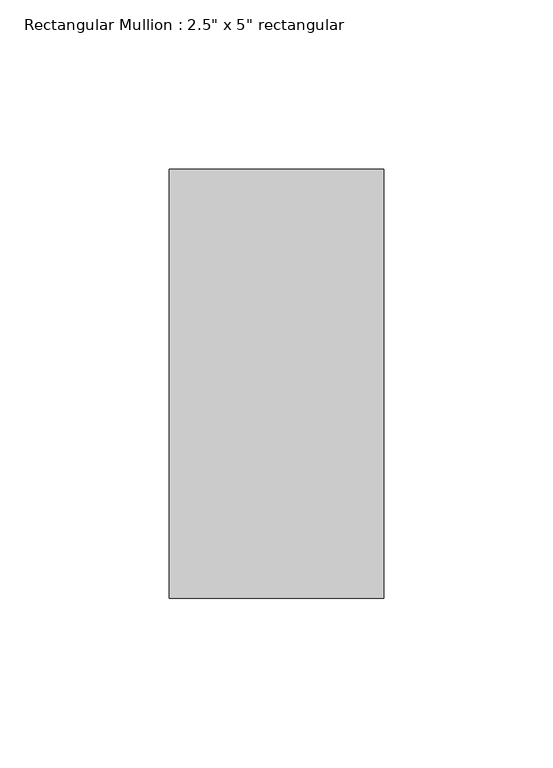
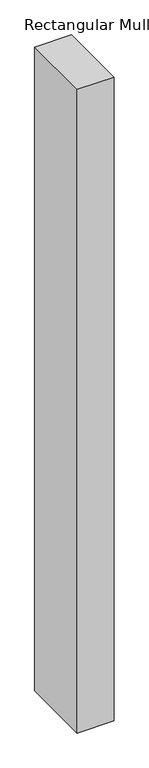
"""IFC4 building model written with IfcOpenShell, lengths in millimetres: member geometry."""

from ifc_helpers import new_model, si_unit, frame, origin, place, context, project, spatial, polyline, outline, extrude, source, transform, mapped, element, save


def member_d9f78736(model_context):
    return source(origin(), model_context, "Body", "SweptSolid", [
        extrude(outline(polyline([(0.0, 63.5), (0.0, -63.5), (-63.5, -63.5), (-63.5, 63.5), (0.0, 63.5)])), frame((0.0, 0.0, -1174.2243728), z_axis=(0.0, 0.0, 1.0), x_axis=(1.0, 0.0, 0.0)), (0.0, 0.0, 1.0), 1174.2243728),
    ])


if __name__ == "__main__":
    model = new_model("IFC4")
    model_context = context("Model", 3, world=origin())
    ifc_project = project(units=[si_unit("LENGTHUNIT", "METRE", prefix="MILLI")], contexts=[model_context])
    site = spatial("IfcSite", under=ifc_project)
    building = spatial("IfcBuilding", under=site)
    placement = place(None, origin())
    member_shape = member_d9f78736(model_context)
    element("IfcMember", 1, ObjectType="Rectangular Mullion : 2.5\" x 5\" rectangular", at=placement, inside=building, context=model_context, shape_type="MappedRepresentation", body=[
        mapped(member_shape, transform((0.0, 0.0, 0.0), x_axis=(1.0, 0.0, 0.0), y_axis=(0.0, 1.0, 0.0), z_axis=(0.0, 0.0, 1.0))),
    ])
    save(model, "model.ifc")

# Revit data of these elements
# Type "Rectangular Mullion : 2.5\" x 5\" rectangular"
#   built-in parameter 1007304 = 0.416667 (stored number, unit not read)
#   built-in parameter 1007301 = 0.104167 (stored number, unit not read)
#   built-in parameter 1007300 = 0.104167 (stored number, unit not read)
# Element 1 (IfcMember, "Rectangular Mullion : 2.5\" x 5\" rectangular")
#   Materials on its faces: "Aluminum"
# Materials
#   "Aluminum": class "Metal", colour RGB 247 247 247, transparency 0, Description = "Aluminum 6061", Cost = 0
